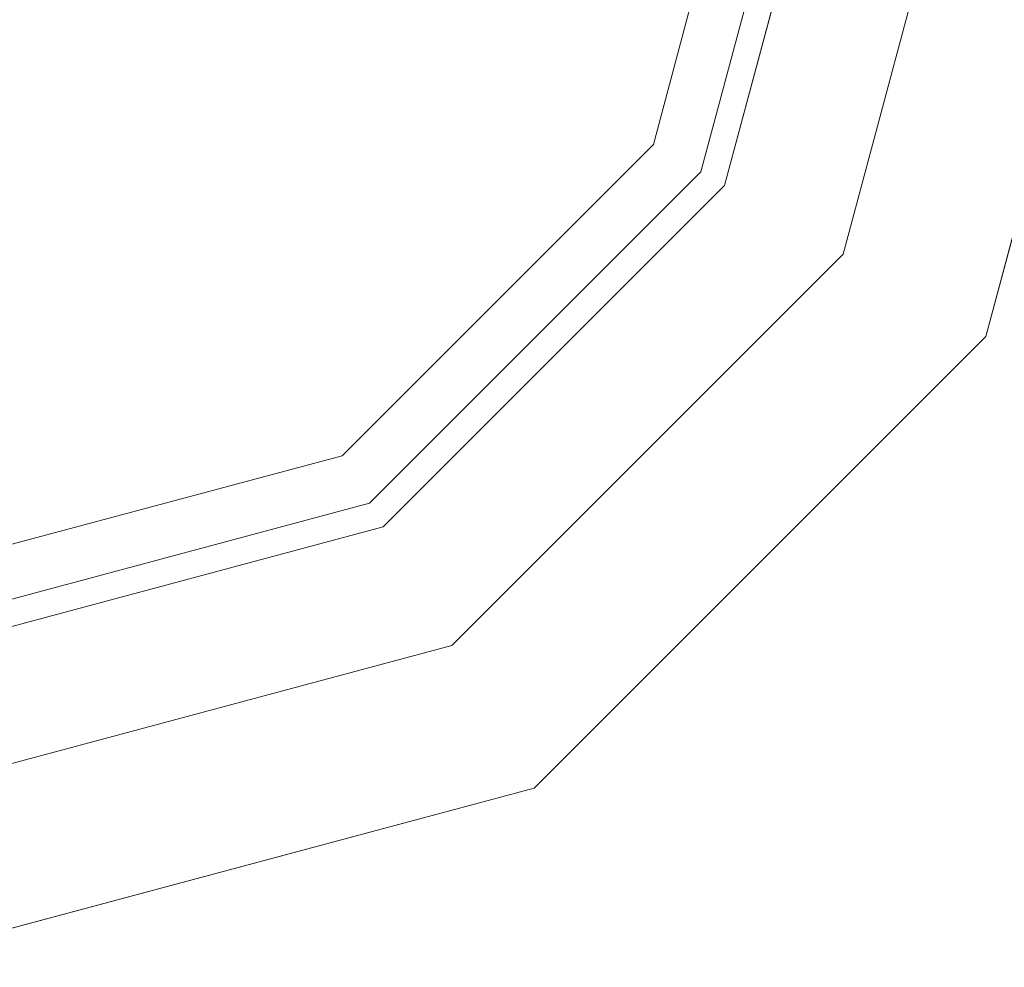
# Model space of a CAD drawing. Units: inches. Extents: x 375 to 1122, y 27 to 1069.
# Tile 96 of 155: x 713.015 to 717.434, y 863.668 to 867.921. Entities that reach past the tile are written whole.
import ezdxf

# ---------------------------------------------------------------- set-up
doc = ezdxf.new("R2010")
doc.units = ezdxf.units.IN
doc.layers.add('A-ANNO-DIMS', color=2, linetype='Continuous', lineweight=18)
doc.layers.add('Furniture', color=30, linetype='Continuous', lineweight=18)
doc.styles.get("Standard").update_dxf_attribs({"font": 'arial.ttf'})
doc.dimstyles.new('ISO-25', dxfattribs={"dimtxt": 12, "dimasz": 2.5, "dimexe": 1.5, "dimexo": 1.5, "dimtad": 1, "dimdec": 1, "dimlunit": 3, "dimtxsty": 'Standard', "dimblk": 'ARCHTICK', "dimcen": 2.5, "dimadec": 0, "dimazin": 0, "dimtfac": 1, "dimtdec": 1, "dimtmove": 0, "dimatfit": 3, "dimfxl": 1.5, "dimfxlon": 1, "dimarcsym": 0})

# ---------------------------------------------------------------- blocks, each defined once
blk = doc.blocks.new('A$C403C54AD')
at = {"linetype": 'ByBlock', "invisible_edges": 5}
for points in [[(1.79578, 0.81008, -0.00874), (1.78654, 0.79408, -0.00874), (1.72651, 0.81017, -0.00874), (1.72651, 0.82864, -0.00874)], [(1.77884, 0.78075, -0.02259), (1.79578, 0.81008, -0.01335), (1.72651, 0.82864, -0.01335), (1.72651, 0.79478, -0.02259)], [(1.78654, 0.79408, -0.00874), (1.7773, 0.77809, -0.01489), (1.72651, 0.7917, -0.01489), (1.72651, 0.81017, -0.00874)], [(1.81715, 0.74244, -0.02259), (1.84648, 0.75938, -0.01335), (1.79578, 0.81008, -0.01335), (1.77884, 0.78075, -0.02259)], [(1.84648, 0.75938, -0.00874), (1.83048, 0.75014, -0.00874), (1.78654, 0.79408, -0.00874), (1.79578, 0.81008, -0.00874)], [(1.77423, 0.77276, -0.03183), (1.77884, 0.78075, -0.02259), (1.72651, 0.79478, -0.02259), (1.72651, 0.78554, -0.03183)], [(1.83048, 0.75014, -0.00874), (1.81449, 0.74091, -0.01489), (1.7773, 0.77809, -0.01489), (1.78654, 0.79408, -0.00874)], [(1.7773, 0.77809, -0.01489), (1.72651, 0.69011, -0.01489), (1.72651, 0.69011, -0.01489), (1.72651, 0.7917, -0.01489)], [(1.80916, 0.73783, -0.03183), (1.81715, 0.74244, -0.02259), (1.77884, 0.78075, -0.02259), (1.77423, 0.77276, -0.03183)], [(1.81449, 0.74091, -0.01489), (1.72651, 0.69011, -0.01489), (1.72651, 0.69011, -0.01489), (1.7773, 0.77809, -0.01489)], [(1.83118, 0.69011, -0.02259), (1.86504, 0.69011, -0.01335), (1.84648, 0.75938, -0.01335), (1.81715, 0.74244, -0.02259)], [(1.86504, 0.69011, -0.00874), (1.84657, 0.69011, -0.00874), (1.83048, 0.75014, -0.00874), (1.84648, 0.75938, -0.00874)], [(1.84657, 0.69011, -0.00874), (1.8281, 0.69011, -0.01489), (1.81449, 0.74091, -0.01489), (1.83048, 0.75014, -0.00874)], [(1.82194, 0.69011, -0.03183), (1.83118, 0.69011, -0.02259), (1.81715, 0.74244, -0.02259), (1.80916, 0.73783, -0.03183)], [(1.8281, 0.69011, -0.01489), (1.72651, 0.69011, -0.01489), (1.72651, 0.69011, -0.01489), (1.81449, 0.74091, -0.01489)]]:
    blk.add_3dface(points, dxfattribs=at)
at = {"linetype": 'ByBlock'}
for points in [[(1.79578, 0.81008, -0.01335), (1.79578, 0.81008, -0.00874), (1.72651, 0.82864, -0.00874), (1.72651, 0.82864, -0.01335)], [(1.84648, 0.75938, -0.01335), (1.84648, 0.75938, -0.00874), (1.79578, 0.81008, -0.00874), (1.79578, 0.81008, -0.01335)], [(1.86504, 0.69011, -0.01335), (1.86504, 0.69011, -0.00874), (1.84648, 0.75938, -0.00874), (1.84648, 0.75938, -0.01335)]]:
    blk.add_3dface(points, dxfattribs=at)
blk = doc.blocks.new('_ArchTick')
at = {"color": 0, "linetype": 'ByBlock', "const_width": 0.15}
blk.add_lwpolyline([(-0.5, -0.5), (0.5, 0.5)], dxfattribs=at)
blk = doc.blocks.new('*D85')
at = {"layer": 'A-ANNO-DIMS', "color": 0, "lineweight": -2, "transparency": 16777216}
for p, q in [((401.5073, 868.5277), (398.5073, 868.5277)), ((400.0073, 814.5277), (400.0073, 868.5277)), ((401.5073, 814.5277), (398.5073, 814.5277))]:
    blk.add_line(p, q, dxfattribs=at)
at = {"layer": 'Defpoints', "color": 0, "transparency": 16777216}
for p in [(400.0073, 868.5277), (845.0073, 868.5277), (845.0073, 814.5277)]:
    blk.add_point(p, dxfattribs=at)
at = {"layer": 'A-ANNO-DIMS', "color": 0, "lineweight": -2, "transparency": 16777216, "xscale": 2.5, "yscale": 2.5, "zscale": 2.5}
for p, rotation in [((400.0073, 868.5277), 90), ((400.0073, 814.5277), 270)]:
    blk.add_blockref('_ArchTick', p, dxfattribs=dict(at, rotation=rotation))
at = {"layer": 'A-ANNO-DIMS', "color": 0, "transparency": 16777216, "insert": (393.2555, 841.5277), "char_height": 12, "attachment_point": 5, "rotation": 90}
blk.add_mtext('4\'-6"', dxfattribs=at)

msp = doc.modelspace()

# ---------------------------------------------------------------- block references
at = {"layer": 'Furniture', "xscale": 39.9918517141215, "yscale": 39.9918517141215, "zscale": 39.9918517141215, "rotation": 270}
msp.add_blockref('A$C403C54AD', (684.9549, 938.3156, 0.024), dxfattribs=at)

# ---------------------------------------------------------------- dimensions: what is measured, and where the dimension line sits
at = {"layer": 'A-ANNO-DIMS'}
dim = msp.add_linear_dim(base=(400.0073, 868.5277), p1=(845.0073, 814.5277), p2=(845.0073, 868.5277), angle=90, dimstyle='ISO-25', override={"dimdec": 1, "dimlfac": 1, "dimrnd": 0, "dimzin": 1, "dimdsep": 46, "dimlunit": 4, "dimfrac": 2}, dxfattribs=at)
dim.commit()
dim.dimension.update_dxf_attribs({"geometry": '*D85', "text_midpoint": (393.2555, 841.5277)})

doc.saveas('drawing.dxf')
